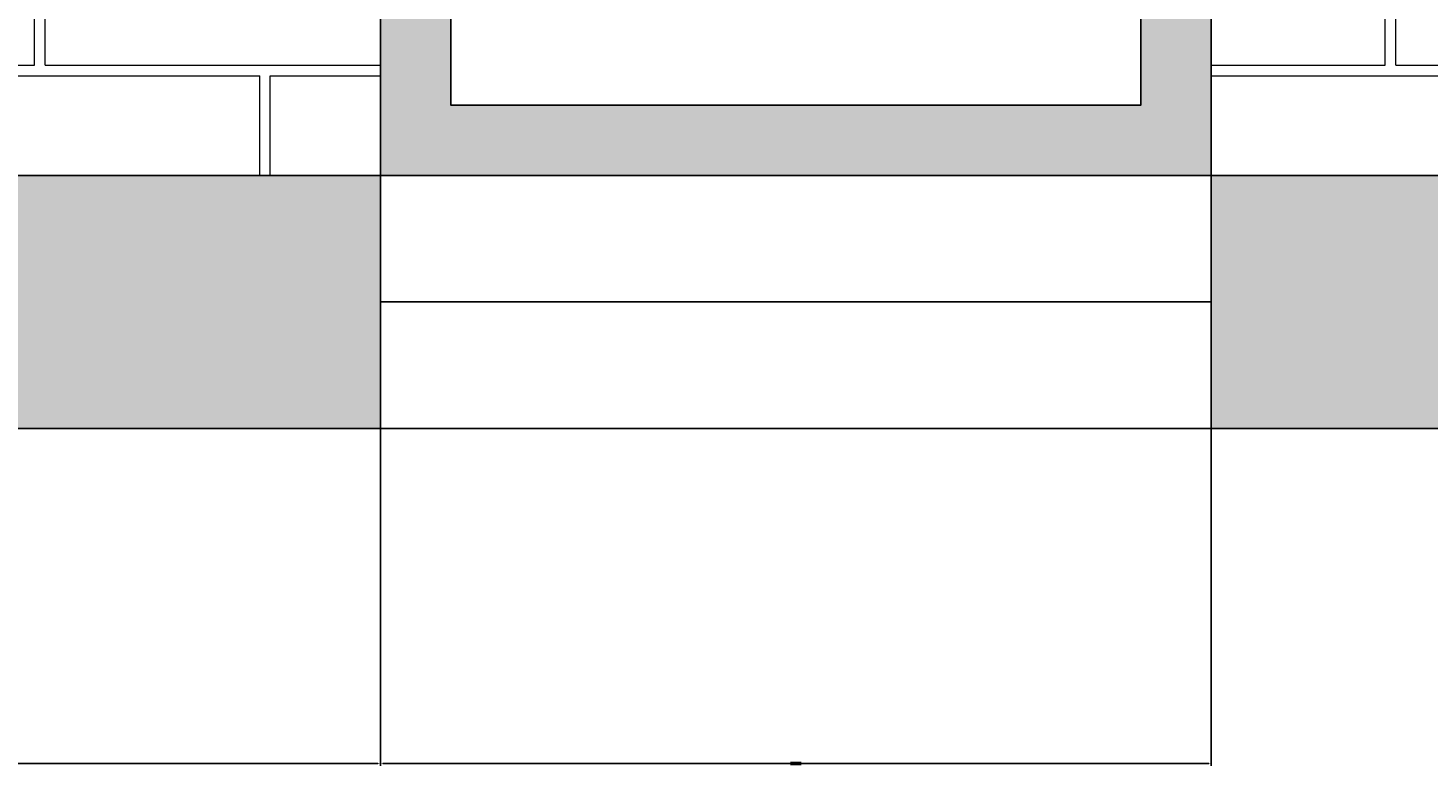
# Model space of a CAD drawing. Units: inches. Extents: x -128 to 854, y -395 to 398.
# Tile 55 of 61: x 467 to 567, y -395 to -343. Entities that reach past the tile are written whole.
import ezdxf

# ---------------------------------------------------------------- set-up
doc = ezdxf.new("R2010")
doc.units = ezdxf.units.IN
doc.header["$MEASUREMENT"] = 0
for name, color, linetype, lineweight in [('A-ANNO-DIMS', 2, 'Continuous', 18), ('A-DOOR', 4, 'Continuous', 25), ('A-ELEV', 3, 'Continuous', 25), ('A-ELEV-PATT', 8, 'Continuous', 13), ('A-FLOR-STRS', 7, 'Continuous', 25)]:
    doc.layers.add(name, color=color, linetype=linetype, lineweight=lineweight)
doc.styles.get("Standard").update_dxf_attribs({"font": 'arial.ttf'})
doc.dimstyles.get("Standard").update_dxf_attribs({"dimtxt": 0.18, "dimasz": 0.18, "dimexe": 0.18, "dimexo": 0.0625, "dimgap": 0.09, "dimtad": 0, "dimtih": 1, "dimtoh": 1, "dimdec": 1, "dimzin": 0, "dimdsep": 46, "dimlunit": 4, "dimtxsty": 'Standard', "dimcen": 0.09, "dimclrd": 1, "dimclre": 2, "dimclrt": 6, "dimadec": 0, "dimazin": 0, "dimtfac": 1, "dimtdec": 1, "dimtofl": 0, "dimtmove": 0, "dimatfit": 3, "dimfxl": 1, "dimtfill": 2, "dimtfillclr": 3, "dimtolj": 1, "dimtzin": 0, "dimarcsym": 0})

# ---------------------------------------------------------------- blocks, each defined once
blk = doc.blocks.new('*D135')
at = {"layer": 'A-ANNO-DIMS', "color": 2, "lineweight": -2, "transparency": 16777216}
for p, q in [((418.28, -371.539), (418.28, -395.456)), ((492.252, -371.539), (492.252, -395.456))]:
    blk.add_line(p, q, dxfattribs=at)
at = {"layer": 'A-ANNO-DIMS', "color": 1, "lineweight": -2, "transparency": 16777216}
for p, q in [((418.46, -395.276), (454.936, -395.276)), ((492.072, -395.276), (455.596, -395.276))]:
    blk.add_line(p, q, dxfattribs=at)
at = {"layer": 'A-ANNO-DIMS', "color": 1, "transparency": 16777216}
for points in [[(418.46, -395.246), (418.46, -395.306), (418.28, -395.276)], [(492.072, -395.246), (492.072, -395.306), (492.252, -395.276)]]:
    blk.add_solid(points, dxfattribs=at)
at = {"layer": 'Defpoints', "color": 0, "transparency": 16777216}
for p in [(418.28, -371.476), (492.252, -371.476), (492.252, -395.276)]:
    blk.add_point(p, dxfattribs=at)
at = {"layer": 'A-ANNO-DIMS', "color": 6, "transparency": 16777216, "insert": (455.266, -395.276), "char_height": 0.18, "attachment_point": 5, "bg_fill": 1, "box_fill_scale": 1.25, "bg_fill_color": 3, "bg_fill_transparency": 0}
blk.add_mtext('\\A1;6\'-2"', dxfattribs=at)
blk = doc.blocks.new('*D136')
at = {"layer": 'A-ANNO-DIMS', "color": 2, "lineweight": -2, "transparency": 16777216}
for p, q in [((492.252, -371.539), (492.252, -395.456)), ((551.307, -371.539), (551.307, -395.456))]:
    blk.add_line(p, q, dxfattribs=at)
at = {"layer": 'A-ANNO-DIMS', "color": 1, "lineweight": -2, "transparency": 16777216}
for p, q in [((492.432, -395.276), (521.377, -395.276)), ((551.127, -395.276), (522.182, -395.276))]:
    blk.add_line(p, q, dxfattribs=at)
at = {"layer": 'A-ANNO-DIMS', "color": 1, "transparency": 16777216}
for points in [[(492.432, -395.246), (492.432, -395.306), (492.252, -395.276)], [(551.127, -395.246), (551.127, -395.306), (551.307, -395.276)]]:
    blk.add_solid(points, dxfattribs=at)
at = {"layer": 'Defpoints', "color": 0, "transparency": 16777216}
for p in [(492.252, -371.476), (551.307, -371.476), (551.307, -395.276)]:
    blk.add_point(p, dxfattribs=at)
at = {"layer": 'A-ANNO-DIMS', "color": 6, "transparency": 16777216, "insert": (521.78, -395.276), "char_height": 0.18, "attachment_point": 5, "bg_fill": 1, "box_fill_scale": 1.25, "bg_fill_color": 3, "bg_fill_transparency": 0}
blk.add_mtext('\\A1;4\'-11"', dxfattribs=at)
blk = doc.blocks.new('*D140')
at = {"layer": 'A-ANNO-DIMS', "color": 2, "lineweight": -2, "transparency": 16777216}
for p, q in [((551.245, -257.476), (346.3, -257.476)), ((551.245, -353.476), (346.3, -353.476))]:
    blk.add_line(p, q, dxfattribs=at)
at = {"layer": 'A-ANNO-DIMS', "color": 1, "lineweight": -2, "transparency": 16777216}
for p, q in [((346.48, -257.656), (346.48, -305.295)), ((346.48, -353.296), (346.48, -305.658))]:
    blk.add_line(p, q, dxfattribs=at)
at = {"layer": 'A-ANNO-DIMS', "color": 1, "transparency": 16777216}
for points in [[(346.45, -257.656), (346.51, -257.656), (346.48, -257.476)], [(346.45, -353.296), (346.51, -353.296), (346.48, -353.476)]]:
    blk.add_solid(points, dxfattribs=at)
at = {"layer": 'Defpoints', "color": 0, "transparency": 16777216}
for p in [(346.48, -257.476), (551.307, -257.476), (551.307, -353.476)]:
    blk.add_point(p, dxfattribs=at)
at = {"layer": 'A-ANNO-DIMS', "color": 6, "transparency": 16777216, "insert": (346.48, -305.476), "char_height": 0.18, "attachment_point": 5, "bg_fill": 1, "box_fill_scale": 1.25, "bg_fill_color": 3, "bg_fill_transparency": 0}
blk.add_mtext('\\A1;8\'-0"', dxfattribs=at)

msp = doc.modelspace()

# ---------------------------------------------------------------- hatches: boundary and pattern name
at = {"layer": 'A-ELEV-PATT'}
h = msp.add_hatch(color=256, dxfattribs=at)
h.dxf.hatch_style = 1
h.paths.add_polyline_path([(418.28, -227.476), (418.28, -233.476), (782.28, -233.476), (782.28, -227.476)])
h.paths.add_polyline_path([(492.252, -257.476), (492.252, -353.476), (551.307, -353.476), (551.307, -257.476)])
h.paths.add_polyline_path([(546.307, -262.476), (546.307, -348.476), (497.252, -348.476), (497.252, -262.476)], flags=16)
h = msp.add_hatch(dxfattribs=at)
h.set_pattern_fill('AR-B816C', color=256, scale=2)
h.set_pattern_definition([(0, (468.407, -10.41), (16, 16), [31.25, -0.75]), (0, (452.407, -9.66), (16, 16), [31.25, -0.75]), (90, (468.407, -10.41), (-16, 16), [-16.75, 15.25]), (90, (467.657, -10.41), (-16, 16), [-16.75, 15.25])])
h.paths.add_polyline_path([(418.28, -353.476), (492.252, -353.476), (492.252, -257.476), (551.307, -257.476), (551.307, -353.476), (782.28, -353.476), (782.28, -233.476), (418.28, -233.476)])
h.paths.add_polyline_path([(668.28, -257.476), (730.28, -257.476), (730.28, -305.476), (668.28, -305.476)], flags=16)
h.paths.add_polyline_path([(673.28, -300.476), (673.28, -262.476), (725.28, -262.476), (725.28, -300.476)], flags=0)
h = msp.add_hatch(dxfattribs=at)
h.set_pattern_fill('AR-CONC', color=256, scale=2)
h.set_pattern_definition([(50, (468.407, -10.41), (14.3452, -1.25504), [1.5, -16.5]), (355, (468.407, -10.41), (-2.77503, 15.04384), [1.2, -13.2]), (100.4514, (469.602, -10.515), (11.57018, 13.7888), [1.2748, -14.02284]), (46.184, (468.407, -6.41), (21.3448, -3.3104), [2.25, -24.75]), (96.6356, (470.186, -6.686), (18.6932, 19.4824), [1.9122, -21.0343]), (351.184, (468.407, -6.41), (18.6932, 19.4824), [1.8, -19.8]), (21, (470.407, -7.41), (11.93814, -8.05238), [1.5, -16.5]), (326, (470.407, -7.41), (4.8663, 14.503), [1.2, -13.2]), (71.4514, (471.402, -8.081), (16.80445, 6.45062), [1.2748, -14.02284]), (37.5, (468.407, -10.4104), (0.243197, 6.657877), [0, -13.04, 0, -13.4, 0, -13.25]), (7.5, (468.407, -10.4104), (5.26139, 7.88823), [0, -7.64, 0, -12.74, 0, -5.05]), (327.5, (463.947, -10.4104), (10.67645, -0.4511), [0, -5, 0, -15.6, 0, -20.7]), (317.5, (461.947, -10.41), (11.66372, 2.0021), [0, -6.5, 0, -10.36, 0, -14.7])])
h.paths.add_polyline_path([(418.28, -353.476), (418.28, -371.476), (492.252, -371.476), (492.252, -353.476)])
h.paths.add_polyline_path([(782.28, -371.476), (782.28, -353.476), (551.307, -353.476), (551.307, -371.476)])

# ---------------------------------------------------------------- linework, layer by layer
at = {"layer": 'A-DOOR'}
for points in [[(492.252, -257.476), (551.307, -257.476), (551.307, -353.476), (492.252, -353.476)], [(497.252, -262.476), (546.307, -262.476), (546.307, -348.476), (497.252, -348.476)]]:
    msp.add_lwpolyline(points, close=True, dxfattribs=at)
at = {"layer": 'A-ELEV'}
for points in [[(418.28, -233.476), (782.28, -233.476), (782.28, -353.476), (418.28, -353.476)], [(418.28, -353.476), (782.28, -353.476), (782.28, -371.476), (418.28, -371.476)]]:
    msp.add_lwpolyline(points, close=True, dxfattribs=at)
at = {"layer": 'A-FLOR-STRS'}
for p, q in [((492.252, -353.476), (551.307, -353.476)), ((492.252, -353.476), (492.252, -371.476)), ((551.307, -353.476), (551.307, -371.476)), ((492.252, -362.476), (551.307, -362.476))]:
    msp.add_line(p, q, dxfattribs=at)

# ---------------------------------------------------------------- dimensions: what is measured, and where the dimension line sits
at = {"layer": 'A-ANNO-DIMS'}
dim = msp.add_linear_dim(base=(346.48, -257.476), p1=(551.307, -353.476), p2=(551.307, -257.476), angle=90, dimstyle='Standard', override={"dimdec": 1, "dimlfac": 1, "dimrnd": 0, "dimzin": 1, "dimdsep": 46, "dimlunit": 4, "dimfrac": 2}, dxfattribs=at)
dim.commit()
dim.dimension.update_dxf_attribs({"geometry": '*D140', "text_midpoint": (346.48, -305.476)})
for base, p1, p2, picture, middle in [((492.252, -395.276), (418.28, -371.476), (492.252, -371.476), '*D135', (455.266, -395.276)), ((551.307, -395.276), (492.252, -371.476), (551.307, -371.476), '*D136', (521.78, -395.276))]:
    dim = msp.add_linear_dim(base=base, p1=p1, p2=p2, dimstyle='Standard', override={"dimdec": 1, "dimlfac": 1, "dimrnd": 0, "dimzin": 1, "dimdsep": 46, "dimlunit": 4, "dimfrac": 2}, dxfattribs=at)
    dim.commit()
    dim.dimension.update_dxf_attribs({"geometry": picture, "text_midpoint": middle})

doc.saveas('drawing.dxf')
